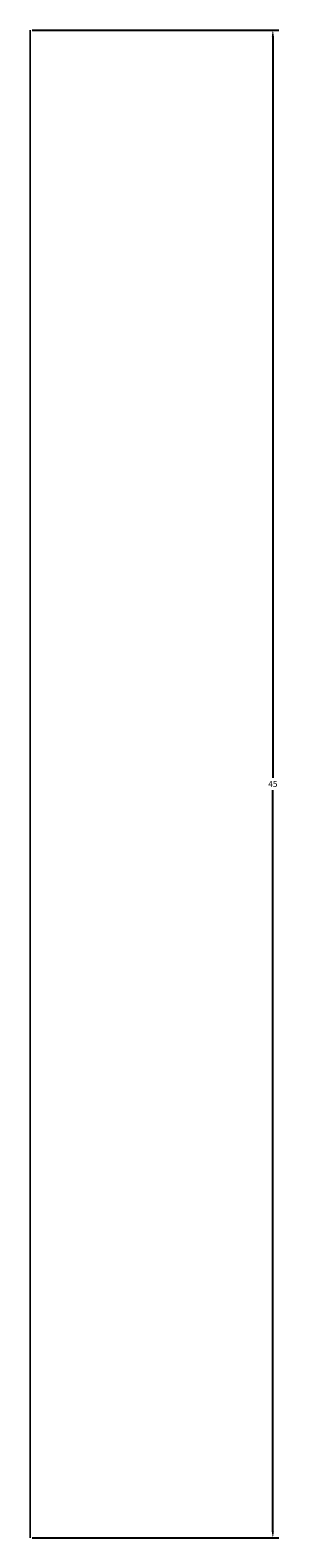
# Model space of a CAD drawing. Units: millimetres. Extents: x 400.8 to 408.2, y 258.2 to 303.2.
import ezdxf

# ---------------------------------------------------------------- set-up
doc = ezdxf.new("R2010")
doc.units = ezdxf.units.MM
doc.layers.add('M-CONS', color=8, linetype='Continuous', lineweight=18)
doc.layers.add('M-DIMS', color=2, linetype='Continuous', lineweight=18)
doc.styles.get("Standard").update_dxf_attribs({"font": 'arial.ttf'})
doc.dimstyles.get("Standard").update_dxf_attribs({"dimtxt": 0.18, "dimasz": 0.18, "dimexe": 0.18, "dimexo": 0.0625, "dimgap": 0.09, "dimtad": 0, "dimtih": 1, "dimtoh": 1, "dimdec": 4, "dimzin": 0, "dimdsep": 46, "dimtxsty": 'Standard', "dimcen": 0.09, "dimadec": 0, "dimazin": 0, "dimtfac": 1, "dimtdec": 4, "dimtofl": 0, "dimtmove": 0, "dimatfit": 3, "dimfxl": 1, "dimtolj": 1, "dimtzin": 0, "dimarcsym": 0})

# ---------------------------------------------------------------- blocks, each defined once
blk = doc.blocks.new('*D1')
at = {"layer": 'Defpoints', "color": 0, "transparency": 16777216}
for p in [(400.807, 303.181), (408.057, 303.181), (400.807, 258.181)]:
    blk.add_point(p, dxfattribs=at)
at = {"layer": 'M-DIMS', "color": 0, "lineweight": -2, "transparency": 16777216}
for p, q in [((400.87, 303.181), (408.237, 303.181)), ((408.057, 303.001), (408.057, 280.862)), ((408.057, 258.361), (408.057, 280.499)), ((400.87, 258.181), (408.237, 258.181))]:
    blk.add_line(p, q, dxfattribs=at)
at = {"layer": 'M-DIMS', "color": 0, "transparency": 16777216}
for points in [[(408.027, 303.001), (408.087, 303.001), (408.057, 303.181)], [(408.027, 258.361), (408.087, 258.361), (408.057, 258.181)]]:
    blk.add_solid(points, dxfattribs=at)
at = {"layer": 'M-DIMS', "color": 0, "transparency": 16777216, "insert": (408.057, 280.681), "char_height": 0.18, "attachment_point": 5}
blk.add_mtext('\\A1;45', dxfattribs=at)

msp = doc.modelspace()

# ---------------------------------------------------------------- linework, layer by layer
at = {"layer": 'M-CONS'}
for p, q in [((400.807, 258.181, 75), (400.807, 303.181, 90)), ((400.807, 303.181, 90), (400.807, 303.181)), ((400.807, 303.181), (400.807, 258.181, 15))]:
    msp.add_line(p, q, dxfattribs=at)

# ---------------------------------------------------------------- dimensions: what is measured, and where the dimension line sits
at = {"layer": 'M-DIMS'}
dim = msp.add_linear_dim(base=(408.057, 303.181), p1=(400.807, 258.181), p2=(400.807, 303.181), angle=90, dimstyle='Standard', override={"dimdec": 0, "dimlfac": 1, "dimrnd": 0, "dimzin": 0, "dimdsep": 46, "dimlunit": 2}, dxfattribs=at)
dim.commit()
dim.dimension.update_dxf_attribs({"geometry": '*D1', "text_midpoint": (408.057, 280.681)})

doc.saveas('drawing.dxf')
